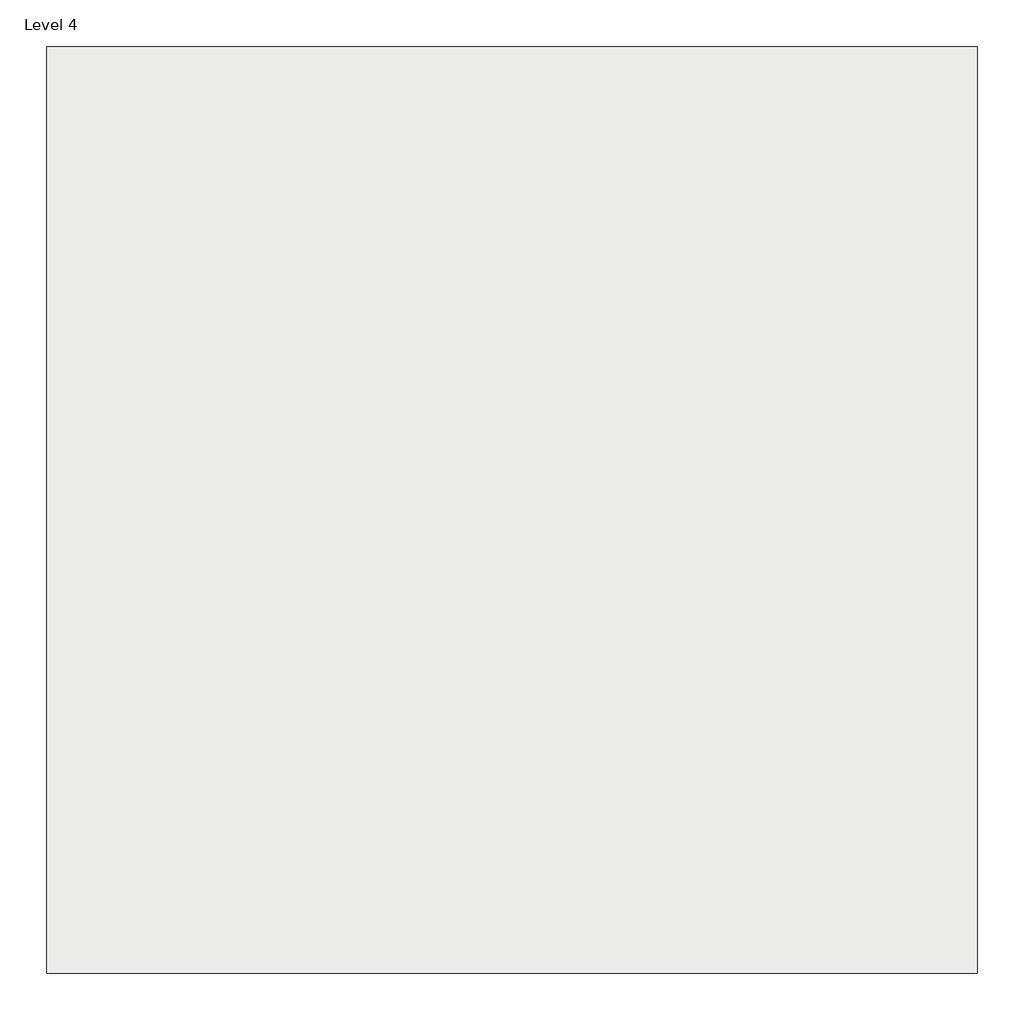
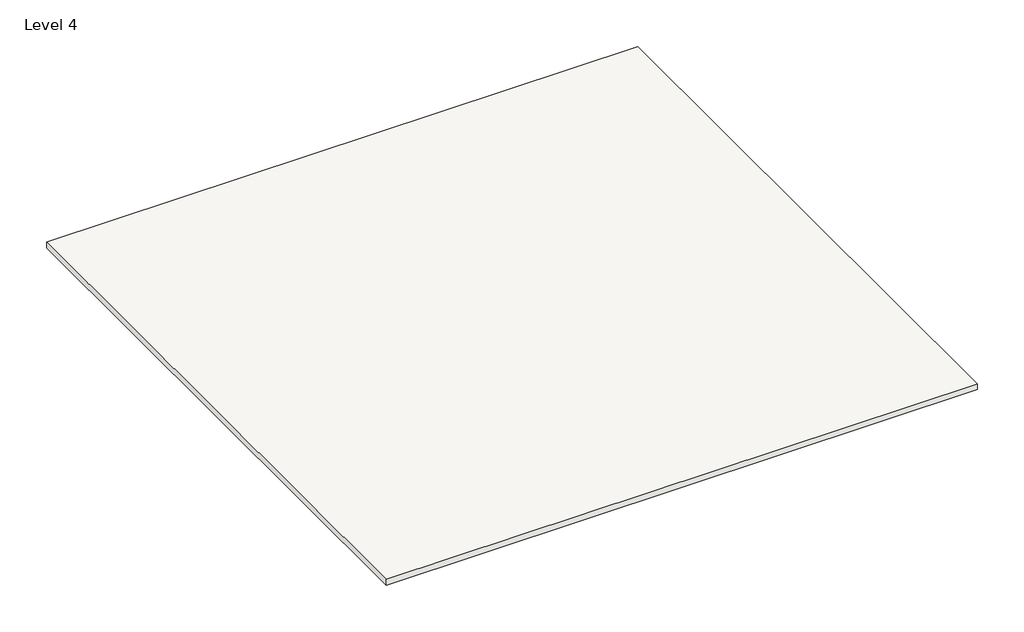
# One storey: 1 roof.
"""IFC4 building model written with IfcOpenShell, lengths in millimetres."""

from ifc_helpers import new_model, si_unit, frame, origin, place, context, project, spatial, polyline, outline, extrude, element, save

model = new_model("IFC4")

# Units and contexts
model_context = context("Model", 3, world=origin())
ifc_project = project(units=[si_unit("LENGTHUNIT", "METRE", prefix="MILLI")], contexts=[model_context])

# Site, building, storey
site = spatial("IfcSite", under=ifc_project)
building = spatial("IfcBuilding", under=site)
storey = spatial("IfcBuildingStorey", under=building, Name="Level 4", Elevation=6324.6)

# Roof
placement = place(None, origin())
element("IfcRoof", 1, ObjectType="Generic - 9\"", at=placement, inside=storey, context=model_context, shape_type="SweptSolid", body=[
    extrude(outline(polyline([(-8934.7629849, 17755.0995758), (12604.4370151, 17755.0995758), (12604.4370151, -3682.5004242), (-8934.7629849, -3682.5004242), (-8934.7629849, 17755.0995758)])), frame((0.0, 0.0, 6324.6), z_axis=(0.0, 0.0, 1.0), x_axis=(1.0, 0.0, 0.0)), (0.0, 0.0, 1.0), 228.6),
])

save(model, "model.ifc")

# Revit data of these elements
# Type "Generic - 9\""
#   Assembly Code = "B1020"
#   Layers, outside or top first: 0' - 9" no material (function 1)
# Element 1 (IfcRoof, "Generic - 9\"")
#   built-in parameter 1001705 = 21.5 (stored number, unit not read)
#   built-in parameter 1001710 = 33615
#   Phase Created = New Construction
#   Materials on its faces: "Default Roof"
# Materials
#   "Default Roof": colour RGB 88 101 114, transparency 0
